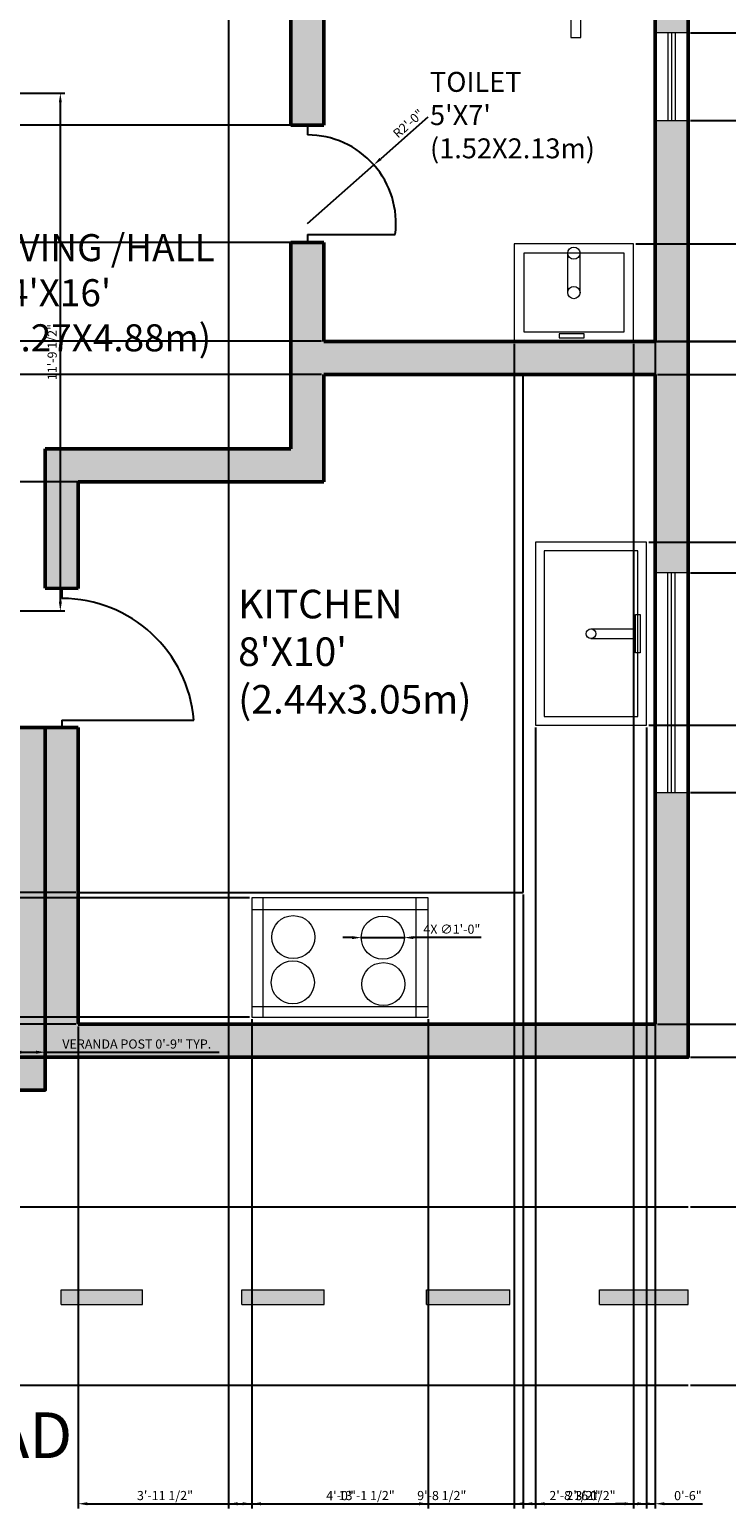
# Model space of a CAD drawing. Units: inches. Extents: x 655 to 1311, y 444 to 1096.
# Tile 2 of 4: x 890 to 1080, y 444 to 848. Entities that reach past the tile are written whole.
import ezdxf

# ---------------------------------------------------------------- set-up
doc = ezdxf.new("R2010")
doc.units = ezdxf.units.IN
for name, color, linetype, lineweight in [('A-ANNO-DIMS', 7, 'Continuous', 18), ('A-ANNO-TEXT', 7, 'Continuous', 18), ('A-AREA-IDEN', 7, 'Continuous', 18), ('A-COLS', 7, 'Continuous', 50), ('A-COLS-PATT', 7, 'Continuous', 13), ('A-EQPM', 8, 'Continuous', 18), ('A-FLOR-CASE', 7, 'Continuous', 25), ('A-FLOR-FIXT', 8, 'Continuous', 18), ('A-WALL', 7, 'Continuous', 50), ('A-WALL-PATT', 7, 'Continuous', 13), ('C-ROAD-MARK', 7, 'Continuous', 13), ('C-ROAD-PATT', 7, 'Continuous', 13)]:
    doc.layers.add(name, color=color, linetype=linetype, lineweight=lineweight)
for name, color, linetype, lineweight, true_color in [('A-DOOR', 251, 'Continuous', 25, 0x636466), ('A-GLAZ', 152, 'Continuous', 18, 0x2776bb), ('C-ROAD', 251, 'Continuous', 25, 0x636466)]:
    doc.layers.add(name, color=color, linetype=linetype, lineweight=lineweight, true_color=true_color)
doc.styles.get("Standard").update_dxf_attribs({"font": 'arial.ttf'})
doc.dimstyles.new('ISO-25', dxfattribs={"dimtxt": 2.5, "dimasz": 2.5, "dimexe": 1.25, "dimexo": 0.625, "dimtad": 1, "dimdec": 0, "dimlunit": 3, "dimtxsty": 'Standard', "dimcen": 2.5, "dimadec": 0, "dimazin": 0, "dimtfac": 1, "dimtdec": 0, "dimtmove": 0, "dimatfit": 3, "dimfxl": 1, "dimarcsym": 0})

# ---------------------------------------------------------------- blocks, each defined once
blk = doc.blocks.new('DOOR-SWING-36IN')
for p, q in [((0, 0), (0, 36)), ((-36, 0), (-33.26, 0)), ((0, 0), (2, 0))]:
    blk.add_line(p, q)
blk.add_arc((2.86, 0), 36.11, 94.5377, 180)
blk = doc.blocks.new('WIN-60IN')
for p, q in [((60, 9), (0, 9)), ((0, 9), (0, 0)), ((60, 0), (60, 9)), ((60, 5.5), (0, 5.5)), ((60, 4.5), (0, 4.5)), ((60, 3.5), (0, 3.5)), ((0, 0), (60, 0))]:
    blk.add_line(p, q)
blk = doc.blocks.new('POST-VERANDA-9IN')
blk.add_line((9, 9), (0, 9))
blk.add_lwpolyline([(0, 9), (0, 0), (9, 0), (9, 9)])
blk = doc.blocks.new('*D16')
at = {"layer": 'A-ANNO-DIMS', "color": 0, "lineweight": -2, "transparency": 16777216}
for p, q in [((884.83, 568.38), (884.83, 570.35)), ((893.83, 568.38), (893.83, 570.35)), ((887.33, 569.1), (891.33, 569.1)), ((893.83, 569.1), (941.28, 569.1))]:
    blk.add_line(p, q, dxfattribs=at)
at = {"layer": 'A-ANNO-DIMS', "color": 0, "transparency": 16777216}
for points in [[(887.33, 569.52), (887.33, 568.69), (884.83, 569.1)], [(891.33, 569.52), (891.33, 568.69), (893.83, 569.1)]]:
    blk.add_solid(points, dxfattribs=at)
at = {"layer": 'Defpoints', "color": 0, "transparency": 16777216}
for p in [(884.83, 567.75), (893.83, 569.1), (893.83, 567.75)]:
    blk.add_point(p, dxfattribs=at)
at = {"layer": 'A-ANNO-DIMS', "color": 0, "transparency": 16777216, "insert": (918.81, 571.02), "char_height": 2.5, "attachment_point": 5}
blk.add_mtext('VERANDA POST 0\'-9" TYP.', dxfattribs=at)
blk = doc.blocks.new('*D22')
at = {"layer": 'A-ANNO-DIMS', "color": 0, "lineweight": -2, "transparency": 16777216}
for p, q in [((943.83, 894.13), (943.83, 444.55)), ((1060.33, 894.13), (1060.33, 444.55)), ((946.33, 445.8), (1057.83, 445.8))]:
    blk.add_line(p, q, dxfattribs=at)
at = {"layer": 'A-ANNO-DIMS', "color": 0, "transparency": 16777216}
for points in [[(946.33, 446.22), (946.33, 445.38), (943.83, 445.8)], [(1057.83, 446.22), (1057.83, 445.38), (1060.33, 445.8)]]:
    blk.add_solid(points, dxfattribs=at)
at = {"layer": 'Defpoints', "color": 0, "transparency": 16777216}
for p in [(943.83, 894.75), (1060.33, 894.75), (1060.33, 445.8)]:
    blk.add_point(p, dxfattribs=at)
at = {"layer": 'A-ANNO-DIMS', "color": 0, "transparency": 16777216, "insert": (1002.08, 447.72), "char_height": 2.5, "attachment_point": 5}
blk.add_mtext('9\'-8 1/2"', dxfattribs=at)
blk = doc.blocks.new('*D25')
at = {"layer": 'A-ANNO-DIMS', "color": 0, "lineweight": -2, "transparency": 16777216}
for p, q in [((1060.96, 885.75), (1102.98, 885.75)), ((1101.73, 765.73), (1101.73, 883.25)), ((1060.96, 763.23), (1102.98, 763.23))]:
    blk.add_line(p, q, dxfattribs=at)
at = {"layer": 'A-ANNO-DIMS', "color": 0, "transparency": 16777216}
for points in [[(1101.32, 883.25), (1102.15, 883.25), (1101.73, 885.75)], [(1101.32, 765.73), (1102.15, 765.73), (1101.73, 763.23)]]:
    blk.add_solid(points, dxfattribs=at)
at = {"layer": 'Defpoints', "color": 0, "transparency": 16777216}
for p in [(1060.33, 885.75), (1101.73, 885.75), (1060.33, 763.23)]:
    blk.add_point(p, dxfattribs=at)
at = {"layer": 'A-ANNO-DIMS', "color": 0, "transparency": 16777216, "insert": (1099.81, 824.49), "char_height": 2.5, "attachment_point": 5, "rotation": 90}
blk.add_mtext('10\'-2 1/2"', dxfattribs=at)
blk = doc.blocks.new('*D26')
at = {"layer": 'A-ANNO-DIMS', "color": 0, "lineweight": -2, "transparency": 16777216}
for p, q in [((1069.96, 847.5), (1102.98, 847.5)), ((1101.73, 826), (1101.73, 845)), ((1069.96, 823.5), (1102.98, 823.5))]:
    blk.add_line(p, q, dxfattribs=at)
at = {"layer": 'A-ANNO-DIMS', "color": 0, "transparency": 16777216}
for points in [[(1101.32, 845), (1102.15, 845), (1101.73, 847.5)], [(1101.32, 826), (1102.15, 826), (1101.73, 823.5)]]:
    blk.add_solid(points, dxfattribs=at)
at = {"layer": 'Defpoints', "color": 0, "transparency": 16777216}
for p in [(1069.33, 847.5), (1101.73, 847.5), (1069.33, 823.5)]:
    blk.add_point(p, dxfattribs=at)
at = {"layer": 'A-ANNO-DIMS', "color": 0, "transparency": 16777216, "insert": (1099.83, 835.5), "char_height": 2.5, "attachment_point": 5, "rotation": 90}
blk.add_mtext('2\'-0"', dxfattribs=at)
blk = doc.blocks.new('*D27')
at = {"layer": 'A-ANNO-DIMS', "color": 0, "lineweight": -2, "transparency": 16777216}
for p, q in [((1069.96, 823.5), (1102.98, 823.5)), ((1101.73, 702.49), (1101.73, 821)), ((1069.96, 699.99), (1102.98, 699.99))]:
    blk.add_line(p, q, dxfattribs=at)
at = {"layer": 'A-ANNO-DIMS', "color": 0, "transparency": 16777216}
for points in [[(1101.32, 821), (1102.15, 821), (1101.73, 823.5)], [(1101.32, 702.49), (1102.15, 702.49), (1101.73, 699.99)]]:
    blk.add_solid(points, dxfattribs=at)
at = {"layer": 'Defpoints', "color": 0, "transparency": 16777216}
for p in [(1069.33, 823.5), (1101.73, 823.5), (1069.33, 699.99)]:
    blk.add_point(p, dxfattribs=at)
at = {"layer": 'A-ANNO-DIMS', "color": 0, "transparency": 16777216, "insert": (1099.81, 761.75), "char_height": 2.5, "attachment_point": 5, "rotation": 90}
blk.add_mtext('10\'-3 1/2"', dxfattribs=at)
blk = doc.blocks.new('*D28')
at = {"layer": 'A-ANNO-DIMS', "color": 0, "lineweight": -2, "transparency": 16777216}
for p, q in [((1069.96, 639.99), (1102.98, 639.99)), ((1101.73, 570.25), (1101.73, 637.49)), ((1069.96, 567.75), (1102.98, 567.75))]:
    blk.add_line(p, q, dxfattribs=at)
at = {"layer": 'A-ANNO-DIMS', "color": 0, "transparency": 16777216}
for points in [[(1101.32, 637.49), (1102.15, 637.49), (1101.73, 639.99)], [(1101.32, 570.25), (1102.15, 570.25), (1101.73, 567.75)]]:
    blk.add_solid(points, dxfattribs=at)
at = {"layer": 'Defpoints', "color": 0, "transparency": 16777216}
for p in [(1069.33, 639.99), (1101.73, 639.99), (1069.33, 567.75)]:
    blk.add_point(p, dxfattribs=at)
at = {"layer": 'A-ANNO-DIMS', "color": 0, "transparency": 16777216, "insert": (1099.83, 603.87), "char_height": 2.5, "attachment_point": 5, "rotation": 90}
blk.add_mtext('6\'-0"', dxfattribs=at)
blk = doc.blocks.new('*D29')
at = {"layer": 'A-ANNO-DIMS', "color": 0, "lineweight": -2, "transparency": 16777216}
for p, q in [((969.27, 790.23), (675.68, 790.23)), ((676.93, 765.73), (676.93, 787.73)), ((969.27, 763.23), (675.68, 763.23))]:
    blk.add_line(p, q, dxfattribs=at)
at = {"layer": 'A-ANNO-DIMS', "color": 0, "transparency": 16777216}
for points in [[(676.52, 787.73), (677.35, 787.73), (676.93, 790.23)], [(676.52, 765.73), (677.35, 765.73), (676.93, 763.23)]]:
    blk.add_solid(points, dxfattribs=at)
at = {"layer": 'Defpoints', "color": 0, "transparency": 16777216}
for p in [(676.93, 790.23), (969.89, 790.23), (969.89, 763.23)]:
    blk.add_point(p, dxfattribs=at)
at = {"layer": 'A-ANNO-DIMS', "color": 0, "transparency": 16777216, "insert": (675.03, 776.73), "char_height": 2.5, "attachment_point": 5, "rotation": 90}
blk.add_mtext('2\'-3"', dxfattribs=at)
blk = doc.blocks.new('*D30')
at = {"layer": 'A-ANNO-DIMS', "color": 0, "lineweight": -2, "transparency": 16777216}
for p, q in [((969.27, 822.23), (675.68, 822.23)), ((676.93, 792.73), (676.93, 819.73)), ((969.27, 790.23), (675.68, 790.23))]:
    blk.add_line(p, q, dxfattribs=at)
at = {"layer": 'A-ANNO-DIMS', "color": 0, "transparency": 16777216}
for points in [[(676.52, 819.73), (677.35, 819.73), (676.93, 822.23)], [(676.52, 792.73), (677.35, 792.73), (676.93, 790.23)]]:
    blk.add_solid(points, dxfattribs=at)
at = {"layer": 'Defpoints', "color": 0, "transparency": 16777216}
for p in [(676.93, 822.23), (969.89, 822.23), (969.89, 790.23)]:
    blk.add_point(p, dxfattribs=at)
at = {"layer": 'A-ANNO-DIMS', "color": 0, "transparency": 16777216, "insert": (675.03, 806.23), "char_height": 2.5, "attachment_point": 5, "rotation": 90}
blk.add_mtext('2\'-8"', dxfattribs=at)
blk = doc.blocks.new('*D31')
at = {"layer": 'A-ANNO-DIMS', "color": 0, "lineweight": -2, "transparency": 16777216}
for p, q in [((1021.86, 762.57), (1021.86, 444.55)), ((1054.47, 762.57), (1054.47, 444.55)), ((1024.36, 445.8), (1051.97, 445.8))]:
    blk.add_line(p, q, dxfattribs=at)
at = {"layer": 'A-ANNO-DIMS', "color": 0, "transparency": 16777216}
for points in [[(1024.36, 446.22), (1024.36, 445.38), (1021.86, 445.8)], [(1051.97, 446.22), (1051.97, 445.38), (1054.47, 445.8)]]:
    blk.add_solid(points, dxfattribs=at)
at = {"layer": 'Defpoints', "color": 0, "transparency": 16777216}
for p in [(1021.86, 763.19), (1054.47, 763.19), (1054.47, 445.8)]:
    blk.add_point(p, dxfattribs=at)
at = {"layer": 'A-ANNO-DIMS', "color": 0, "transparency": 16777216, "insert": (1038.16, 447.72), "char_height": 2.5, "attachment_point": 5}
blk.add_mtext('2\'-8 1/2"', dxfattribs=at)
blk = doc.blocks.new('*D32')
at = {"layer": 'A-ANNO-DIMS', "color": 0, "lineweight": -2, "transparency": 16777216}
for p, q in [((1055.1, 789.89), (1102.98, 789.89)), ((1101.73, 765.69), (1101.73, 787.39)), ((1055.1, 763.19), (1102.98, 763.19))]:
    blk.add_line(p, q, dxfattribs=at)
at = {"layer": 'A-ANNO-DIMS', "color": 0, "transparency": 16777216}
for points in [[(1101.32, 787.39), (1102.15, 787.39), (1101.73, 789.89)], [(1101.32, 765.69), (1102.15, 765.69), (1101.73, 763.19)]]:
    blk.add_solid(points, dxfattribs=at)
at = {"layer": 'Defpoints', "color": 0, "transparency": 16777216}
for p in [(1054.47, 789.89), (1101.73, 789.89), (1054.47, 763.19)]:
    blk.add_point(p, dxfattribs=at)
at = {"layer": 'A-ANNO-DIMS', "color": 0, "transparency": 16777216, "insert": (1099.81, 776.54), "char_height": 2.5, "attachment_point": 5, "rotation": 90}
blk.add_mtext('2\'-2 1/2"', dxfattribs=at)
blk = doc.blocks.new('*D33')
at = {"layer": 'A-ANNO-DIMS', "color": 0, "lineweight": -2, "transparency": 16777216}
for p, q in [((1054.47, 762.57), (1054.47, 444.55)), ((1060.33, 762.6), (1060.33, 444.55)), ((1051.97, 445.8), (1049.47, 445.8)), ((1054.47, 445.8), (1060.33, 445.8)), ((1062.83, 445.8), (1073.23, 445.8))]:
    blk.add_line(p, q, dxfattribs=at)
at = {"layer": 'A-ANNO-DIMS', "color": 0, "transparency": 16777216}
for points in [[(1051.97, 446.22), (1051.97, 445.38), (1054.47, 445.8)], [(1062.83, 446.22), (1062.83, 445.38), (1060.33, 445.8)]]:
    blk.add_solid(points, dxfattribs=at)
at = {"layer": 'Defpoints', "color": 0, "transparency": 16777216}
for p in [(1054.47, 763.19), (1060.33, 763.23), (1060.33, 445.8)]:
    blk.add_point(p, dxfattribs=at)
at = {"layer": 'A-ANNO-DIMS', "color": 0, "transparency": 16777216, "insert": (1069.28, 447.7), "char_height": 2.5, "attachment_point": 5}
blk.add_mtext('0\'-6"', dxfattribs=at)
blk = doc.blocks.new('*D36')
at = {"layer": 'A-ANNO-DIMS', "color": 0, "lineweight": -2, "transparency": 16777216}
for p, q in [((1060.96, 754.19), (1102.98, 754.19)), ((1101.73, 579.25), (1101.73, 751.69)), ((1060.96, 576.75), (1102.98, 576.75))]:
    blk.add_line(p, q, dxfattribs=at)
at = {"layer": 'A-ANNO-DIMS', "color": 0, "transparency": 16777216}
for points in [[(1101.32, 751.69), (1102.15, 751.69), (1101.73, 754.19)], [(1101.32, 579.25), (1102.15, 579.25), (1101.73, 576.75)]]:
    blk.add_solid(points, dxfattribs=at)
at = {"layer": 'Defpoints', "color": 0, "transparency": 16777216}
for p in [(1060.33, 754.19), (1101.73, 754.19), (1060.33, 576.75)]:
    blk.add_point(p, dxfattribs=at)
at = {"layer": 'A-ANNO-DIMS', "color": 0, "transparency": 16777216, "insert": (1099.81, 665.47), "char_height": 2.5, "attachment_point": 5, "rotation": 90}
blk.add_mtext('14\'-9 1/2"', dxfattribs=at)
blk = doc.blocks.new('*D37')
at = {"layer": 'A-ANNO-DIMS', "color": 0, "lineweight": -2, "transparency": 16777216}
for p, q in [((902.83, 576.13), (902.83, 444.55)), ((1060.33, 576.13), (1060.33, 444.55)), ((905.33, 445.8), (1057.83, 445.8))]:
    blk.add_line(p, q, dxfattribs=at)
at = {"layer": 'A-ANNO-DIMS', "color": 0, "transparency": 16777216}
for points in [[(905.33, 446.22), (905.33, 445.38), (902.83, 445.8)], [(1057.83, 446.22), (1057.83, 445.38), (1060.33, 445.8)]]:
    blk.add_solid(points, dxfattribs=at)
at = {"layer": 'Defpoints', "color": 0, "transparency": 16777216}
for p in [(902.83, 576.75), (1060.33, 576.75), (1060.33, 445.8)]:
    blk.add_point(p, dxfattribs=at)
at = {"layer": 'A-ANNO-DIMS', "color": 0, "transparency": 16777216, "insert": (981.58, 447.72), "char_height": 2.5, "attachment_point": 5}
blk.add_mtext('13\'-1 1/2"', dxfattribs=at)
blk = doc.blocks.new('*D38')
at = {"layer": 'A-ANNO-DIMS', "color": 0, "lineweight": -2, "transparency": 16777216}
for p, q in [((969.27, 754.19), (675.68, 754.19)), ((676.93, 727.35), (676.93, 751.69)), ((969.27, 724.85), (675.68, 724.85))]:
    blk.add_line(p, q, dxfattribs=at)
at = {"layer": 'A-ANNO-DIMS', "color": 0, "transparency": 16777216}
for points in [[(676.52, 751.69), (677.35, 751.69), (676.93, 754.19)], [(676.52, 727.35), (677.35, 727.35), (676.93, 724.85)]]:
    blk.add_solid(points, dxfattribs=at)
at = {"layer": 'Defpoints', "color": 0, "transparency": 16777216}
for p in [(676.93, 754.19), (969.89, 754.19), (969.89, 724.85)]:
    blk.add_point(p, dxfattribs=at)
at = {"layer": 'A-ANNO-DIMS', "color": 0, "transparency": 16777216, "insert": (675.01, 739.52), "char_height": 2.5, "attachment_point": 5, "rotation": 90}
blk.add_mtext('2\'-5 1/2"', dxfattribs=at)
blk = doc.blocks.new('*D39')
at = {"layer": 'A-ANNO-DIMS', "color": 0, "lineweight": -2, "transparency": 16777216}
for p, q in [((902.21, 612.75), (675.68, 612.75)), ((676.93, 579.25), (676.93, 610.25)), ((902.21, 576.75), (675.68, 576.75))]:
    blk.add_line(p, q, dxfattribs=at)
at = {"layer": 'A-ANNO-DIMS', "color": 0, "transparency": 16777216}
for points in [[(676.52, 610.25), (677.35, 610.25), (676.93, 612.75)], [(676.52, 579.25), (677.35, 579.25), (676.93, 576.75)]]:
    blk.add_solid(points, dxfattribs=at)
at = {"layer": 'Defpoints', "color": 0, "transparency": 16777216}
for p in [(676.93, 612.75), (902.83, 612.75), (902.83, 576.75)]:
    blk.add_point(p, dxfattribs=at)
at = {"layer": 'A-ANNO-DIMS', "color": 0, "transparency": 16777216, "insert": (675.03, 594.75), "char_height": 2.5, "attachment_point": 5, "rotation": 90}
blk.add_mtext('3\'-0"', dxfattribs=at)
blk = doc.blocks.new('*D40')
at = {"layer": 'A-ANNO-DIMS', "color": 0, "lineweight": -2, "transparency": 16777216}
for p, q in [((1060.33, 639.37), (1060.33, 444.55)), ((1024.33, 612.13), (1024.33, 444.55)), ((1026.83, 445.8), (1057.83, 445.8))]:
    blk.add_line(p, q, dxfattribs=at)
at = {"layer": 'A-ANNO-DIMS', "color": 0, "transparency": 16777216}
for points in [[(1026.83, 446.22), (1026.83, 445.38), (1024.33, 445.8)], [(1057.83, 446.22), (1057.83, 445.38), (1060.33, 445.8)]]:
    blk.add_solid(points, dxfattribs=at)
at = {"layer": 'Defpoints', "color": 0, "transparency": 16777216}
for p in [(1060.33, 639.99), (1024.33, 612.75), (1060.33, 445.8)]:
    blk.add_point(p, dxfattribs=at)
at = {"layer": 'A-ANNO-DIMS', "color": 0, "transparency": 16777216, "insert": (1042.33, 447.7), "char_height": 2.5, "attachment_point": 5}
blk.add_mtext('3\'-0"', dxfattribs=at)
blk = doc.blocks.new('*D41')
at = {"layer": 'A-ANNO-DIMS', "color": 0, "lineweight": -2, "transparency": 16777216}
for p, q in [((1027.67, 657.81), (1027.67, 444.55)), ((1057.97, 657.81), (1057.97, 444.55)), ((1030.17, 445.8), (1055.47, 445.8))]:
    blk.add_line(p, q, dxfattribs=at)
at = {"layer": 'A-ANNO-DIMS', "color": 0, "transparency": 16777216}
for points in [[(1030.17, 446.22), (1030.17, 445.38), (1027.67, 445.8)], [(1055.47, 446.22), (1055.47, 445.38), (1057.97, 445.8)]]:
    blk.add_solid(points, dxfattribs=at)
at = {"layer": 'Defpoints', "color": 0, "transparency": 16777216}
for p in [(1027.67, 658.43), (1057.97, 658.43), (1057.97, 445.8)]:
    blk.add_point(p, dxfattribs=at)
at = {"layer": 'A-ANNO-DIMS', "color": 0, "transparency": 16777216, "insert": (1042.82, 447.72), "char_height": 2.5, "attachment_point": 5}
blk.add_mtext('2\'-6 1/2"', dxfattribs=at)
blk = doc.blocks.new('*D42')
at = {"layer": 'A-ANNO-DIMS', "color": 0, "lineweight": -2, "transparency": 16777216}
for p, q in [((1058.6, 708.34), (1102.98, 708.34)), ((1101.73, 660.93), (1101.73, 705.84)), ((1058.6, 658.43), (1102.98, 658.43))]:
    blk.add_line(p, q, dxfattribs=at)
at = {"layer": 'A-ANNO-DIMS', "color": 0, "transparency": 16777216}
for points in [[(1101.32, 705.84), (1102.15, 705.84), (1101.73, 708.34)], [(1101.32, 660.93), (1102.15, 660.93), (1101.73, 658.43)]]:
    blk.add_solid(points, dxfattribs=at)
at = {"layer": 'Defpoints', "color": 0, "transparency": 16777216}
for p in [(1057.97, 708.34), (1101.73, 708.34), (1057.97, 658.43)]:
    blk.add_point(p, dxfattribs=at)
at = {"layer": 'A-ANNO-DIMS', "color": 0, "transparency": 16777216, "insert": (1099.85, 683.38), "char_height": 2.5, "attachment_point": 5, "rotation": 90}
blk.add_mtext('4\'-2"', dxfattribs=at)
blk = doc.blocks.new('*D43')
at = {"layer": 'A-ANNO-DIMS', "color": 0, "lineweight": -2, "transparency": 16777216}
for p, q in [((1060.96, 754.19), (1102.98, 754.19)), ((1101.73, 710.84), (1101.73, 751.69)), ((1058.6, 708.34), (1102.98, 708.34))]:
    blk.add_line(p, q, dxfattribs=at)
at = {"layer": 'A-ANNO-DIMS', "color": 0, "transparency": 16777216}
for points in [[(1101.32, 751.69), (1102.15, 751.69), (1101.73, 754.19)], [(1101.32, 710.84), (1102.15, 710.84), (1101.73, 708.34)]]:
    blk.add_solid(points, dxfattribs=at)
at = {"layer": 'Defpoints', "color": 0, "transparency": 16777216}
for p in [(1060.33, 754.19), (1101.73, 754.19), (1057.97, 708.34)]:
    blk.add_point(p, dxfattribs=at)
at = {"layer": 'A-ANNO-DIMS', "color": 0, "transparency": 16777216, "insert": (1099.83, 731.26), "char_height": 2.5, "attachment_point": 5, "rotation": 90}
blk.add_mtext('3\'-10"', dxfattribs=at)
blk = doc.blocks.new('*D44')
at = {"layer": 'A-ANNO-DIMS', "color": 0, "lineweight": -2, "transparency": 16777216}
for p, q in [((950.2, 578.09), (950.2, 444.55)), ((998.39, 578.09), (998.39, 444.55)), ((952.7, 445.8), (995.89, 445.8))]:
    blk.add_line(p, q, dxfattribs=at)
at = {"layer": 'A-ANNO-DIMS', "color": 0, "transparency": 16777216}
for points in [[(952.7, 446.22), (952.7, 445.38), (950.2, 445.8)], [(995.89, 446.22), (995.89, 445.38), (998.39, 445.8)]]:
    blk.add_solid(points, dxfattribs=at)
at = {"layer": 'Defpoints', "color": 0, "transparency": 16777216}
for p in [(950.2, 578.71), (998.39, 578.71), (998.39, 445.8)]:
    blk.add_point(p, dxfattribs=at)
at = {"layer": 'A-ANNO-DIMS', "color": 0, "transparency": 16777216, "insert": (974.3, 447.7), "char_height": 2.5, "attachment_point": 5}
blk.add_mtext('4\'-0"', dxfattribs=at)
blk = doc.blocks.new('*D45')
at = {"layer": 'A-ANNO-DIMS', "color": 0, "lineweight": -2, "transparency": 16777216}
for p, q in [((949.58, 611.29), (675.68, 611.29)), ((676.93, 581.21), (676.93, 608.79)), ((949.58, 578.71), (675.68, 578.71))]:
    blk.add_line(p, q, dxfattribs=at)
at = {"layer": 'A-ANNO-DIMS', "color": 0, "transparency": 16777216}
for points in [[(676.52, 608.79), (677.35, 608.79), (676.93, 611.29)], [(676.52, 581.21), (677.35, 581.21), (676.93, 578.71)]]:
    blk.add_solid(points, dxfattribs=at)
at = {"layer": 'Defpoints', "color": 0, "transparency": 16777216}
for p in [(676.93, 611.29), (950.2, 611.29), (950.2, 578.71)]:
    blk.add_point(p, dxfattribs=at)
at = {"layer": 'A-ANNO-DIMS', "color": 0, "transparency": 16777216, "insert": (675.01, 595), "char_height": 2.5, "attachment_point": 5, "rotation": 90}
blk.add_mtext('2\'-8 1/2"', dxfattribs=at)
blk = doc.blocks.new('*D46')
at = {"layer": 'A-ANNO-DIMS', "color": 0, "lineweight": -2, "transparency": 16777216}
for p, q in [((902.83, 576.13), (902.83, 444.55)), ((950.2, 578.09), (950.2, 444.55)), ((905.33, 445.8), (947.7, 445.8))]:
    blk.add_line(p, q, dxfattribs=at)
at = {"layer": 'A-ANNO-DIMS', "color": 0, "transparency": 16777216}
for points in [[(905.33, 446.22), (905.33, 445.38), (902.83, 445.8)], [(947.7, 446.22), (947.7, 445.38), (950.2, 445.8)]]:
    blk.add_solid(points, dxfattribs=at)
at = {"layer": 'Defpoints', "color": 0, "transparency": 16777216}
for p in [(950.2, 578.71), (902.83, 576.75), (950.2, 445.8)]:
    blk.add_point(p, dxfattribs=at)
at = {"layer": 'A-ANNO-DIMS', "color": 0, "transparency": 16777216, "insert": (926.52, 447.72), "char_height": 2.5, "attachment_point": 5}
blk.add_mtext('3\'-11 1/2"', dxfattribs=at)
blk = doc.blocks.new('*D52')
at = {"layer": 'A-ANNO-DIMS', "color": 0, "lineweight": -2, "transparency": 16777216}
for p, q in [((1069.96, 526.9), (1102.98, 526.9)), ((1101.73, 480.7), (1101.73, 524.4)), ((1069.96, 478.2), (1102.98, 478.2))]:
    blk.add_line(p, q, dxfattribs=at)
at = {"layer": 'A-ANNO-DIMS', "color": 0, "transparency": 16777216}
for points in [[(1101.32, 524.4), (1102.15, 524.4), (1101.73, 526.9)], [(1101.32, 480.7), (1102.15, 480.7), (1101.73, 478.2)]]:
    blk.add_solid(points, dxfattribs=at)
at = {"layer": 'Defpoints', "color": 0, "transparency": 16777216}
for p in [(1069.33, 526.9), (1101.73, 526.9), (1069.33, 478.2)]:
    blk.add_point(p, dxfattribs=at)
at = {"layer": 'A-ANNO-DIMS', "color": 0, "transparency": 16777216, "insert": (1099.81, 502.55), "char_height": 2.5, "attachment_point": 5, "rotation": 90}
blk.add_mtext('4\'-0 1/2"', dxfattribs=at)
blk = doc.blocks.new('*D56')
at = {"layer": 'A-ANNO-DIMS', "color": 0, "lineweight": -2, "transparency": 16777216}
for p, q in [((866.17, 830.95), (899.19, 830.95)), ((897.94, 828.45), (897.94, 692.12)), ((866.17, 689.62), (899.19, 689.62))]:
    blk.add_line(p, q, dxfattribs=at)
at = {"layer": 'A-ANNO-DIMS', "color": 0, "transparency": 16777216}
for points in [[(897.53, 828.45), (898.36, 828.45), (897.94, 830.95)], [(897.53, 692.12), (898.36, 692.12), (897.94, 689.62)]]:
    blk.add_solid(points, dxfattribs=at)
at = {"layer": 'Defpoints', "color": 0, "transparency": 16777216}
for p in [(865.54, 830.95), (865.54, 689.62), (897.94, 689.62)]:
    blk.add_point(p, dxfattribs=at)
at = {"layer": 'A-ANNO-DIMS', "color": 0, "transparency": 16777216, "insert": (896.03, 760.29), "char_height": 2.5, "attachment_point": 5, "rotation": 90}
blk.add_mtext('11\'-9 1/2"', dxfattribs=at)
blk = doc.blocks.new('*D64')
at = {"layer": 'A-ANNO-DIMS', "color": 0, "lineweight": -2, "transparency": 16777216}
for p, q in [((998.26, 824.42), (985.4, 813.07)), ((965.39, 795.41), (983.52, 811.41))]:
    blk.add_line(p, q, dxfattribs=at)
at = {"layer": 'A-ANNO-DIMS', "color": 0, "transparency": 16777216}
blk.add_solid([(985.12, 813.38), (985.67, 812.76), (983.52, 811.41)], dxfattribs=at)
at = {"layer": 'Defpoints', "color": 0, "transparency": 16777216}
for p in [(983.52, 811.41), (965.39, 795.41)]:
    blk.add_point(p, dxfattribs=at)
at = {"layer": 'A-ANNO-DIMS', "color": 0, "transparency": 16777216, "insert": (993.15, 822.44), "char_height": 2.5, "attachment_point": 5, "rotation": 41.4406}
blk.add_mtext('R2\'-0"', dxfattribs=at)
blk = doc.blocks.new('*D67')
at = {"layer": 'A-ANNO-DIMS', "color": 0, "lineweight": -2, "transparency": 16777216}
for p, q in [((977.6, 600.4), (975.1, 600.4)), ((980.1, 600.4), (991.86, 600.39)), ((1012.81, 600.39), (994.36, 600.39))]:
    blk.add_line(p, q, dxfattribs=at)
at = {"layer": 'A-ANNO-DIMS', "color": 0, "transparency": 16777216}
for points in [[(977.6, 600.81), (977.6, 599.98), (980.1, 600.4)], [(994.36, 600.81), (994.36, 599.98), (991.86, 600.39)]]:
    blk.add_solid(points, dxfattribs=at)
at = {"layer": 'Defpoints', "color": 0, "transparency": 16777216}
for p in [(980.1, 600.4), (991.86, 600.39)]:
    blk.add_point(p, dxfattribs=at)
at = {"layer": 'A-ANNO-DIMS', "color": 0, "transparency": 16777216, "insert": (1004.83, 602.37), "char_height": 2.5, "attachment_point": 5, "rotation": 359.9972}
blk.add_mtext('4X ∅1\'-0"', dxfattribs=at)

msp = doc.modelspace()

# ---------------------------------------------------------------- hatches: boundary and pattern name
at = {"layer": 'A-COLS-PATT'}
h = msp.add_hatch(color=256, dxfattribs=at)
h.dxf.hatch_style = 1
h.paths.add_polyline_path([(718.33, 558.75), (718.33, 567.75), (709.33, 567.75), (709.33, 558.75)])
h.paths.add_polyline_path([(893.83, 567.75), (884.83, 567.75), (884.83, 558.75), (893.83, 558.75)])
h.paths.add_polyline_path([(875.1, 756.19), (944.53, 756.19), (944.53, 796.18), (875.1, 796.18)], flags=9)
h.paths.add_polyline_path([(997.04, 810.04), (1045.86, 810.04), (1045.86, 839.51), (997.04, 839.51)], flags=9)
h.paths.add_polyline_path([(949.57, 925.87), (1005.17, 925.87), (1005.17, 959.21), (949.57, 959.21)], flags=9)
h.paths.add_polyline_path([(762.7, 920.37), (822.54, 920.37), (822.54, 956.25), (762.7, 956.25)], flags=9)
at = {"layer": 'A-WALL-PATT'}
h = msp.add_hatch(color=256, dxfattribs=at)
h.dxf.hatch_style = 1
h.paths.add_polyline_path([(969.89, 885.75), (1060.33, 885.75), (1060.33, 847.5), (1069.33, 847.5), (1069.33, 1047.75), (1007.08, 1047.75), (1007.08, 1038.75), (1060.33, 1038.75), (1060.33, 894.75), (943.83, 894.75), (943.83, 885.75), (960.89, 885.75), (960.89, 822.23), (969.89, 822.23)])
h.paths.add_polyline_path([(969.89, 780.75), (969.89, 790.23), (960.89, 790.23), (960.89, 733.85), (893.83, 733.85), (893.83, 695.8), (902.83, 695.71), (902.83, 724.85), (969.89, 724.85), (969.89, 754.19), (1060.33, 754.19), (1060.33, 699.99), (1069.33, 699.99), (1069.33, 823.5), (1060.33, 823.5), (1060.33, 763.19), (969.89, 763.19)])
h.paths.add_polyline_path([(947.08, 1047.75), (821.27, 1047.75), (821.27, 1038.75), (884.83, 1038.75), (884.83, 976.7), (884.83, 894.75), (872.83, 894.75), (872.83, 885.75), (905.83, 885.75), (905.83, 894.75), (893.83, 894.75), (893.83, 1038.75), (921.42, 1038.75), (947.08, 1038.75)])
h.paths.add_polyline_path([(761.27, 1047.75), (709.33, 1047.75), (709.33, 648.75), (736.08, 648.75), (736.08, 657.75), (718.33, 657.75), (718.33, 885.75), (834.83, 885.75), (834.83, 894.75), (718.33, 894.75), (718.33, 1038.75), (761.27, 1038.75)])
h.paths.add_polyline_path([(822.83, 657.75), (796.08, 657.75), (796.08, 648.75), (822.83, 648.75)], flags=17)
h.paths.add_polyline_path([(893.83, 657.75), (860.83, 657.75), (860.83, 648.75), (884.83, 648.75), (884.83, 567.75), (893.83, 567.75)])
h.paths.add_polyline_path([(902.83, 657.75), (893.83, 657.75), (893.83, 567.75), (1069.33, 567.75), (1069.33, 639.99), (1060.33, 639.99), (1060.33, 576.75), (902.83, 576.75)])
at = {"layer": 'C-ROAD-PATT'}
h = msp.add_hatch(color=256, dxfattribs=at)
h.dxf.hatch_style = 1
h.paths.add_polyline_path([(735.91, 504.18), (709.33, 504.18), (709.33, 500.25), (735.91, 500.25)])
h.paths.add_polyline_path([(779.58, 504.18), (777.58, 504.18), (758.08, 504.18), (758.08, 500.25), (777.58, 500.25), (779.58, 500.25)])
h.paths.add_polyline_path([(825.58, 504.18), (802.58, 504.18), (802.58, 500.25), (825.58, 500.25)])
h.paths.add_polyline_path([(874.18, 504.18), (849.64, 504.18), (849.64, 500.25), (874.18, 500.25)])
h.paths.add_polyline_path([(969.96, 504.18), (947.46, 504.18), (947.46, 500.25), (969.96, 500.25)])
h.paths.add_polyline_path([(920.36, 504.18), (898.19, 504.18), (898.19, 500.25), (920.36, 500.25)])
h.paths.add_polyline_path([(1020.63, 504.18), (997.93, 504.18), (997.93, 500.25), (1020.63, 500.25)])
h.paths.add_polyline_path([(1069.33, 504.18), (1045.17, 504.18), (1045.17, 500.25), (1069.33, 500.25)])

# ---------------------------------------------------------------- linework, layer by layer
at = {"layer": 'A-DOOR'}
for p, q in [((965.39, 822.23), (965.39, 819.59)), ((965.39, 792.41), (989.39, 792.41)), ((965.39, 792.41), (965.39, 790.23))]:
    msp.add_line(p, q, dxfattribs=at)
msp.add_arc((965.39, 795.41), 24.19, 352.8794, 90, dxfattribs=at)
at = {"layer": 'A-EQPM'}
for p, q in [((998.39, 611.29), (950.2, 611.29)), ((950.2, 611.29), (950.2, 578.71)), ((953.2, 611.29), (953.2, 578.71)), ((995.12, 578.71), (995.12, 611.29)), ((998.39, 578.71), (998.39, 611.29)), ((998.39, 608), (950.2, 608)), ((950.2, 581.62), (998.39, 581.62)), ((950.2, 578.71), (998.39, 578.71))]:
    msp.add_line(p, q, dxfattribs=at)
for centre in [(961.55, 600.53), (985.98, 600.4), (961.41, 588.18), (986.13, 587.7)]:
    msp.add_circle(centre, 5.88, dxfattribs=at)
at = {"layer": 'A-FLOR-CASE'}
for p, q in [((1024.33, 612.75), (1024.33, 754.19)), ((902.83, 612.75), (1024.33, 612.75))]:
    msp.add_line(p, q, dxfattribs=at)
at = {"layer": 'A-FLOR-FIXT'}
for p, q in [((1036.49, 776.54), (1036.49, 787.29)), ((1039.84, 776.54), (1039.84, 787.29)), ((1042.82, 684.69), (1054.94, 684.69)), ((1042.82, 682.08), (1054.94, 682.08))]:
    msp.add_line(p, q, dxfattribs=at)
for points in [[(1037.33, 846.23), (1040.06, 846.23), (1040.06, 878.53), (1037.33, 878.53)], [(1021.86, 763.19), (1054.47, 763.19), (1054.47, 789.89), (1021.86, 789.89)], [(1024.46, 765.79), (1051.87, 765.79), (1051.87, 787.29), (1024.46, 787.29)], [(1034.17, 764.14), (1040.94, 764.14), (1040.94, 765.23), (1034.17, 765.23)], [(1027.67, 658.43), (1057.97, 658.43), (1057.97, 708.34), (1027.67, 708.34)], [(1030.03, 660.79), (1055.62, 660.79), (1055.62, 705.98), (1030.03, 705.98)], [(1056.29, 678.15), (1054.94, 678.15), (1054.94, 688.61), (1056.29, 688.61)]]:
    msp.add_lwpolyline(points, close=True, dxfattribs=at)
for centre, radius in [((1038.16, 787.29), 1.67), ((1038.16, 776.54), 1.67), ((1042.82, 683.38), 1.31)]:
    msp.add_circle(centre, radius, dxfattribs=at)
at = {"layer": 'A-GLAZ'}
for p, q in [((1063.83, 847.5), (1063.83, 823.5)), ((1064.83, 847.5), (1064.83, 823.5)), ((1065.83, 847.5), (1065.83, 823.5))]:
    msp.add_line(p, q, dxfattribs=at)
msp.add_lwpolyline([(1060.33, 847.5), (1060.33, 823.5), (1069.33, 823.5), (1069.33, 847.5)], close=True, dxfattribs=at)
at = {"layer": 'A-WALL'}
for p, q in [((960.89, 822.23), (960.89, 885.75)), ((969.89, 822.23), (969.89, 885.75)), ((1060.33, 763.19), (1060.33, 885.75)), ((960.89, 822.23), (969.89, 822.23)), ((960.89, 733.85), (960.89, 790.23)), ((960.89, 790.23), (969.89, 790.23)), ((969.89, 772.23), (969.89, 790.23)), ((969.89, 763.19), (969.89, 780.75)), ((969.89, 763.19), (969.89, 763.23)), ((1060.33, 763.19), (969.89, 763.19)), ((1060.33, 763.19), (1060.33, 763.23)), ((1060.33, 754.19), (969.89, 754.19)), ((969.89, 724.85), (969.89, 754.19)), ((1060.33, 576.75), (1060.33, 754.19)), ((893.83, 695.8), (893.83, 733.85)), ((893.83, 733.85), (960.89, 733.85)), ((902.83, 724.85), (969.89, 724.85)), ((902.83, 695.71), (902.83, 724.85)), ((902.83, 695.71), (893.83, 695.8)), ((860.83, 657.75), (902.83, 657.75)), ((893.83, 657.75), (893.83, 567.75)), ((902.83, 657.75), (902.83, 576.75)), ((902.83, 576.75), (1060.33, 576.75))]:
    msp.add_line(p, q, dxfattribs=at)
msp.add_lwpolyline([(893.83, 567.75), (1069.33, 567.75), (1069.33, 1047.75), (709.33, 1047.75), (709.33, 567.75)], dxfattribs=at)
at = {"layer": 'C-ROAD'}
for p, q in [((825.58, 526.9), (1069.33, 526.9)), ((825.58, 478.2), (1069.33, 478.2))]:
    msp.add_line(p, q, dxfattribs=at)
at = {"layer": 'C-ROAD-MARK'}
for p, q in [((898.19, 500.25), (898.19, 504.18)), ((898.19, 504.18), (920.36, 504.18)), ((920.36, 500.25), (920.36, 504.18)), ((947.46, 500.25), (947.46, 504.18)), ((947.46, 504.18), (969.96, 504.18)), ((969.96, 500.25), (969.96, 504.18)), ((997.93, 500.25), (997.93, 504.18)), ((997.93, 504.18), (1020.63, 504.18)), ((1020.63, 500.25), (1020.63, 504.18)), ((1045.17, 500.25), (1045.17, 504.18)), ((1045.17, 504.18), (1069.33, 504.18)), ((1069.33, 500.25), (1069.33, 504.18)), ((898.19, 500.25), (920.36, 500.25)), ((947.46, 500.25), (969.96, 500.25)), ((997.93, 500.25), (1020.63, 500.25)), ((1045.17, 500.25), (1069.33, 500.25))]:
    msp.add_line(p, q, dxfattribs=at)

# ---------------------------------------------------------------- block references
at = {"layer": 'A-COLS'}
msp.add_blockref('POST-VERANDA-9IN', (884.83, 558.75), dxfattribs=at)
at = {"layer": 'A-DOOR', "rotation": 270.0000000000005}
msp.add_blockref('DOOR-SWING-36IN', (898.37, 659.75), dxfattribs=at)
at = {"layer": 'A-GLAZ', "rotation": 269.9999999999999}
msp.add_blockref('WIN-60IN', (1060.33, 699.99), dxfattribs=at)

# ---------------------------------------------------------------- texts
at = {"layer": 'A-ANNO-TEXT', "insert": (855.63, 470.76), "char_height": 12.499, "attachment_point": 1}
msp.add_mtext_dynamic_manual_height_columns('ROAD', width=237.3876, gutter_width=58.61, heights=[0], dxfattribs=at)
at = {"layer": 'A-AREA-IDEN', "attachment_point": 1}
for s, width, gutter_width, insert, char_height in [("TOILET\\P5'X7'\\P(1.52X2.13m)", 87.0922, 27.23, (998.86, 836.8), 5.4456), ("LIVING /HALL\\P14'X16'\\P(4.27X4.88m)", 351.6756, 36.92, (878.07, 792.5), 7.3846), ("KITCHEN\\P8'X10'\\P(2.44x3.05m)", 179.5703, 39.01, (946.49, 695.38), 7.8014)]:
    msp.add_mtext_dynamic_manual_height_columns(s, width=width, gutter_width=gutter_width, heights=[0], dxfattribs=dict(at, insert=insert, char_height=char_height))

# ---------------------------------------------------------------- dimensions: what is measured, and where the dimension line sits
at = {"layer": 'A-ANNO-DIMS'}
for base, p1, p2, picture, middle in [((1060.33, 445.8), (943.83, 894.75), (1060.33, 894.75), '*D22', (1002.08, 447.72)), ((1054.47, 445.8), (1021.86, 763.19), (1054.47, 763.19), '*D31', (1038.16, 447.72)), ((1060.33, 445.8), (1054.47, 763.19), (1060.33, 763.23), '*D33', (1069.28, 447.7)), ((1057.97, 445.8), (1027.67, 658.43), (1057.97, 658.43), '*D41', (1042.82, 447.72)), ((1060.33, 445.8), (1024.33, 612.75), (1060.33, 639.99), '*D40', (1042.33, 447.7)), ((950.2, 445.8), (902.83, 576.75), (950.2, 578.71), '*D46', (926.52, 447.72)), ((998.39, 445.8), (950.2, 578.71), (998.39, 578.71), '*D44', (974.3, 447.7)), ((1060.33, 445.8), (902.83, 576.75), (1060.33, 576.75), '*D37', (981.58, 447.72))]:
    dim = msp.add_linear_dim(base=base, p1=p1, p2=p2, dimstyle='ISO-25', override={"dimdec": 1, "dimlfac": 1, "dimrnd": 0, "dimzin": 1, "dimdsep": 46, "dimlunit": 4, "dimfrac": 2}, dxfattribs=at)
    dim.commit()
    dim.dimension.update_dxf_attribs({"geometry": picture, "text_midpoint": middle})
for base, p1, p2, angle, picture, middle in [((1101.73, 885.75), (1060.33, 763.23), (1060.33, 885.75), 90, '*D25', (1099.81, 824.49)), ((1101.73, 847.5), (1069.33, 823.5), (1069.33, 847.5), 90, '*D26', (1099.83, 835.5)), ((897.94, 689.62), (865.54, 830.95), (865.54, 689.62), 270, '*D56', (896.03, 760.29)), ((676.93, 822.23), (969.89, 790.23), (969.89, 822.23), 90, '*D30', (675.03, 806.23)), ((1101.73, 823.5), (1069.33, 699.99), (1069.33, 823.5), 90, '*D27', (1099.81, 761.75)), ((676.93, 790.23), (969.89, 763.23), (969.89, 790.23), 90, '*D29', (675.03, 776.73)), ((1101.73, 789.89), (1054.47, 763.19), (1054.47, 789.89), 90, '*D32', (1099.81, 776.54)), ((676.93, 754.19), (969.89, 724.85), (969.89, 754.19), 90, '*D38', (675.01, 739.52)), ((1101.7326, 754.1916), (1057.971, 708.3354), (1060.3326, 754.1916), 90, '*D43', (1099.8303, 731.2635)), ((1101.73, 754.19), (1060.33, 576.75), (1060.33, 754.19), 90, '*D36', (1099.81, 665.47)), ((1101.73, 708.34), (1057.97, 658.43), (1057.97, 708.34), 90, '*D42', (1099.85, 683.38)), ((1101.73, 639.99), (1069.33, 567.75), (1069.33, 639.99), 90, '*D28', (1099.83, 603.87)), ((676.93, 611.29), (950.2, 578.71), (950.2, 611.29), 90, '*D45', (675.01, 595)), ((676.93, 612.75), (902.83, 576.75), (902.83, 612.75), 90, '*D39', (675.03, 594.75)), ((1101.73, 526.9), (1069.33, 478.2), (1069.33, 526.9), 90, '*D52', (1099.81, 502.55))]:
    dim = msp.add_linear_dim(base=base, p1=p1, p2=p2, angle=angle, dimstyle='ISO-25', override={"dimdec": 1, "dimlfac": 1, "dimrnd": 0, "dimzin": 1, "dimdsep": 46, "dimlunit": 4, "dimfrac": 2}, dxfattribs=at)
    dim.commit()
    dim.dimension.update_dxf_attribs({"geometry": picture, "text_midpoint": middle})
dim = msp.add_radius_dim(center=(965.39, 795.41), mpoint=(983.52, 811.41), dimstyle='ISO-25', override={"dimdec": 1, "dimlfac": 1, "dimrnd": 0, "dimzin": 1, "dimdsep": 46, "dimlunit": 4, "dimfrac": 2}, dxfattribs=at)
dim.commit()
dim.dimension.update_dxf_attribs({"geometry": '*D64', "text_midpoint": (994.4, 821.02), "dimtype": 164})
dim = msp.add_diameter_dim_2p(p1=(980.1, 600.4), p2=(991.86, 600.39), text='4X <>', dimstyle='ISO-25', override={"dimdec": 1, "dimlfac": 1, "dimrnd": 0, "dimzin": 1, "dimdsep": 46, "dimlunit": 4, "dimfrac": 2}, dxfattribs=at)
dim.commit()
dim.dimension.update_dxf_attribs({"geometry": '*D67', "text_midpoint": (1004.83, 600.39), "dimtype": 163})
dim = msp.add_linear_dim(base=(893.83, 569.1), p1=(884.83, 567.75), p2=(893.83, 567.75), text='VERANDA POST <> TYP.', dimstyle='ISO-25', override={"dimdec": 1, "dimlfac": 1, "dimrnd": 0, "dimzin": 1, "dimdsep": 46, "dimlunit": 4, "dimfrac": 2}, dxfattribs=at)
dim.commit()
dim.dimension.update_dxf_attribs({"geometry": '*D16', "text_midpoint": (918.81, 571.02)})

doc.saveas('drawing.dxf')
